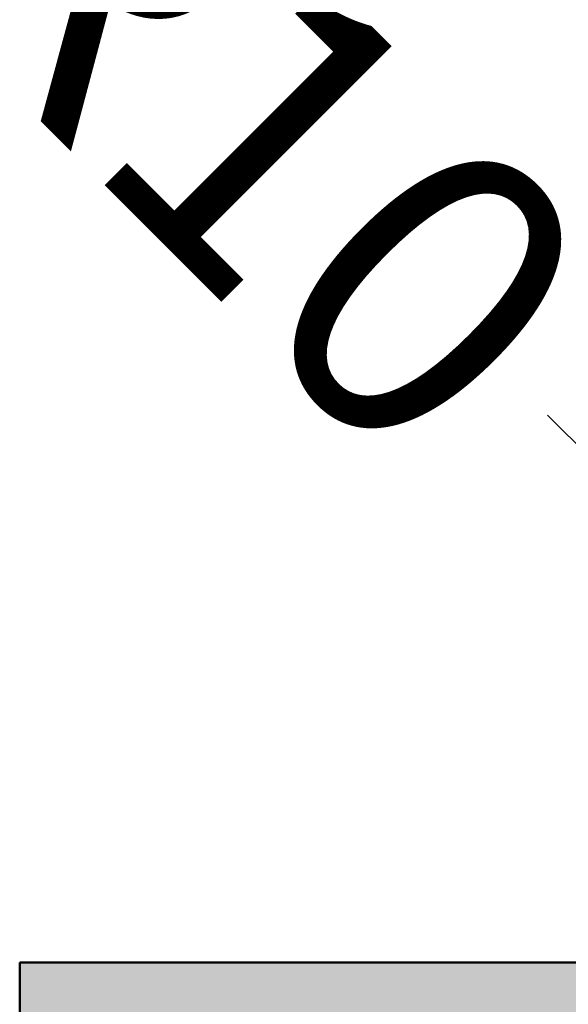
# Model space of a CAD drawing. Units: millimetres. Extents: x 0 to 2267, y 0 to 1823.
# Tile 13 of 256: x 1506 to 1519, y 1116 to 1139. Entities that reach past the tile are written whole.
import ezdxf

# ---------------------------------------------------------------- set-up
doc = ezdxf.new("R2010")
doc.units = ezdxf.units.MM
doc.header["$MEASUREMENT"] = 0
for name, color, linetype, lineweight in [('M-DIMS', 2, 'Continuous', 25), ('M-HATC', 252, 'Continuous', 18), ('M-OUTL', 7, 'Continuous', 50)]:
    doc.layers.add(name, color=color, linetype=linetype, lineweight=lineweight)
doc.styles.get("Standard").update_dxf_attribs({"font": 'arial.ttf'})
doc.dimstyles.get("Standard").update_dxf_attribs({"dimtxt": 7, "dimasz": 4, "dimexe": 0.18, "dimexo": 0.0625, "dimgap": 0.09, "dimtad": 0, "dimdec": 0, "dimzin": 0, "dimdsep": 46, "dimtxsty": 'Standard', "dimcen": 0.09, "dimadec": 0, "dimazin": 0, "dimtfac": 1, "dimtdec": 0, "dimtofl": 0, "dimtmove": 0, "dimatfit": 3, "dimfxl": 1, "dimtolj": 1, "dimtzin": 0, "dimarcsym": 0})

# ---------------------------------------------------------------- blocks, each defined once
blk = doc.blocks.new('*D28')
at = {"layer": 'Defpoints', "color": 0, "transparency": 16777216}
for p in [(1523.858, 1124.488), (1530.929, 1117.417)]:
    blk.add_point(p, dxfattribs=at)
at = {"layer": 'M-DIMS', "color": 0, "lineweight": -2, "transparency": 16777216}
for p, q in [((1518.201, 1130.145), (1521.029, 1127.317)), ((1530.839, 1117.417), (1531.019, 1117.417)), ((1530.929, 1117.327), (1530.929, 1117.507))]:
    blk.add_line(p, q, dxfattribs=at)
at = {"layer": 'M-DIMS', "color": 0, "transparency": 16777216}
blk.add_solid([(1521.501, 1127.788), (1520.558, 1126.845), (1523.858, 1124.488)], dxfattribs=at)
at = {"layer": 'M-DIMS', "color": 0, "transparency": 16777216, "insert": (1504.949, 1143.397), "char_height": 7, "attachment_point": 5, "rotation": 314.9998}
blk.add_mtext('\\A1;27X R10', dxfattribs=at)

msp = doc.modelspace()

# ---------------------------------------------------------------- hatches: boundary and pattern name
at = {"layer": 'M-HATC'}
h = msp.add_hatch(color=256, dxfattribs=at)
h.dxf.hatch_style = 1
h.paths.add_polyline_path([(2065.771, 1618.062, 0.236068), (2055.771, 1638.062), (1381.087, 1638.062, 0.236068), (1371.087, 1618.062), (1371.087, 1603.062), (2055.771, 1603.062), (2065.771, 1603.062)])
h.paths.add_polyline_path([(2062.772, 1550.296), (2062.772, 1560.296), (1374.086, 1560.296), (1374.086, 1550.296), (1374.086, 1540.296), (1384.086, 1540.296), (1389.086, 1540.296), (2062.772, 1540.296)])
h.paths.add_polyline_path([(1930.929, 1282.766), (1505.929, 1282.766), (1587.628, 1235.597, 0.131652), (1600.128, 1232.247), (1836.73, 1232.247, 0.131652), (1849.23, 1235.597)])
h.paths.add_polyline_path([(1930.929, 1117.417), (1905.929, 1117.417), (1505.929, 1117.417), (1505.929, 1077.417), (1930.929, 1077.417)])
h = msp.add_hatch(color=256, dxfattribs=at)
h.dxf.hatch_style = 1
h.paths.add_polyline_path([(2055.771, 1603.062), (1381.087, 1603.062), (1381.087, 1598.062), (2055.771, 1598.062)])
h.paths.add_polyline_path([(2055.771, 1598.062), (1381.087, 1598.062), (1381.087, 1593.062), (2055.771, 1593.062)])
h.paths.add_polyline_path([(2051.307, 1536.761), (1385.55, 1536.761), (1385.55, 1526.761), (1387.55, 1526.761), (1388.537, 1525.053), (1385.332, 1521.233), (1385.332, 1521.223), (2050.254, 1522.749), (2048.321, 1525.053), (2049.307, 1526.761), (2051.307, 1526.761)])
edge = h.paths.add_edge_path()
edge.add_arc((1847.535, 1379.149), 135, 222.60306, 222.89085, ccw=False)
edge.add_line((1748.166, 1287.766), (1683.092, 1287.766))
edge.add_arc((1583.724, 1379.149), 135, 317.10915, 317.39694, ccw=False)
edge.add_arc((1678.969, 1290.671), 5, 222.8909, 317.1091, ccw=False)
edge.add_arc((1774.213, 1379.149), 135, 222.60306, 222.89085, ccw=False)
edge.add_line((1674.845, 1287.766), (1609.771, 1287.766))
edge.add_arc((1510.403, 1379.149), 135, 317.10915, 317.39694, ccw=False)
edge.add_arc((1605.647, 1290.671), 5, 222.8909, 317.1091, ccw=False)
edge.add_arc((1700.892, 1379.149), 135, 222.60306, 222.89085, ccw=False)
edge.add_line((1601.524, 1287.766), (1536.45, 1287.766))
edge.add_arc((1437.081, 1379.149), 135, 317.10915, 317.39694, ccw=False)
edge.add_arc((1532.326, 1290.671), 5, 222.8909, 317.1091, ccw=False)
edge.add_arc((1627.571, 1379.149), 135, 222.60306, 222.89085, ccw=False)
edge.add_line((1528.203, 1287.766), (1505.929, 1287.766))
edge.add_spline(control_points=[(1505.929, 1287.766), (1504.262, 1287.766), (1504.262, 1282.766), (1505.929, 1282.766)], knot_values=[0, 0, 0, 0, 5, 5, 5, 5], degree=3, periodic=0)
edge.add_line((1505.929, 1282.766), (1930.929, 1282.766))
edge.add_spline(control_points=[(1930.929, 1282.766), (1932.596, 1282.766), (1932.596, 1287.766), (1930.929, 1287.766)], knot_values=[0, 0, 0, 0, 5, 5, 5, 5], degree=3, periodic=0)
edge.add_line((1930.929, 1287.766), (1903.056, 1287.766))
edge.add_arc((1803.688, 1379.149), 135, 317.10915, 317.39694, ccw=False)
edge.add_arc((1898.932, 1290.671), 5, 222.8909, 317.1091, ccw=False)
edge.add_arc((1994.177, 1379.149), 135, 222.60306, 222.89085, ccw=False)
edge.add_line((1894.809, 1287.766), (1829.735, 1287.766))
edge.add_arc((1730.366, 1379.149), 135, 317.10915, 317.39694, ccw=False)
edge.add_arc((1825.611, 1290.671), 5, 222.8909, 317.1091, ccw=False)
edge.add_arc((1920.856, 1379.149), 135, 222.60306, 222.89085, ccw=False)
edge.add_line((1821.487, 1287.766), (1756.413, 1287.766))
edge.add_arc((1657.045, 1379.149), 135, 317.10915, 317.39694, ccw=False)
edge.add_arc((1752.29, 1290.671), 5, 222.8909, 317.1091, ccw=False)
edge = h.paths.add_edge_path()
edge.add_spline(control_points=[(1843.429, 1227.247), (1845.096, 1227.247), (1845.096, 1232.247), (1843.429, 1232.247)], knot_values=[0, 0, 0, 0, 5, 5, 5, 5], degree=3, periodic=0)
edge.add_line((1843.429, 1232.247), (1593.429, 1232.247))
edge.add_spline(control_points=[(1593.429, 1232.247), (1591.762, 1232.247), (1591.762, 1227.247), (1593.429, 1227.247)], knot_values=[0, 0, 0, 0, 5, 5, 5, 5], degree=3, periodic=0)
edge.add_line((1593.429, 1227.247), (1843.429, 1227.247))
h.paths.add_polyline_path([(1905.929, 1127.417), (1530.929, 1127.417, 0.414214), (1520.929, 1117.417), (1530.929, 1117.417), (1915.929, 1117.417, 0.414214)])
edge = h.paths.add_edge_path()
edge.add_arc((1397.086, 1498.408), 12.73, 90.7821, 190.8787, ccw=False)
edge.add_line((1396.912, 1511.136), (1428.01, 1511.349))
edge.add_line((1428.01, 1511.349), (1433.01, 1511.349))
edge.add_line((1433.01, 1511.349), (1434.439, 1511.349))
edge.add_arc((1419.474, 1498.08), 20, 41.561, 74.0821)
edge.add_line((1424.959, 1517.314), (1399.935, 1517.256))
edge.add_spline(control_points=[(1399.931, 1517.256), (1399.884, 1517.213), (1399.833, 1517.169), (1399.777, 1517.124)], knot_values=[11.567499, 11.567499, 11.567499, 11.567499, 11.814249, 11.814249, 11.814249, 11.814249], degree=3, periodic=0)
edge.add_spline(control_points=[(1399.633, 1517.01), (1399.583, 1516.972), (1399.531, 1516.934), (1399.476, 1516.895)], knot_values=[11.167718, 11.167718, 11.167718, 11.167718, 11.365188, 11.365188, 11.365188, 11.365188], degree=3, periodic=0)
edge.add_spline(control_points=[(1399.34, 1516.8), (1399.151, 1516.672), (1398.938, 1516.538), (1398.704, 1516.399)], knot_values=[10.376405, 10.376405, 10.376405, 10.376405, 11.00994, 11.00994, 11.00994, 11.00994], degree=3, periodic=0)
edge.add_spline(control_points=[(1398.657, 1516.372), (1398.579, 1516.326), (1398.498, 1516.28), (1398.415, 1516.233)], knot_values=[10.125175, 10.125175, 10.125175, 10.125175, 10.334406, 10.334406, 10.334406, 10.334406], degree=3, periodic=0)
edge.add_spline(control_points=[(1398.264, 1516.149), (1398.196, 1516.111), (1398.126, 1516.073), (1398.055, 1516.035)], knot_values=[9.832246, 9.832246, 9.832246, 9.832246, 9.999658, 9.999658, 9.999658, 9.999658], degree=3, periodic=0)
edge.add_spline(control_points=[(1397.999, 1516.005), (1397.731, 1515.862), (1397.446, 1515.717), (1397.147, 1515.571)], knot_values=[9.161808, 9.161808, 9.161808, 9.161808, 9.787769, 9.787769, 9.787769, 9.787769], degree=3, periodic=0)
edge.add_spline(control_points=[(1397.147, 1515.571), (1396.842, 1515.423), (1396.522, 1515.274), (1396.191, 1515.126)], knot_values=[8.524455, 8.524455, 8.524455, 8.524455, 9.161808, 9.161808, 9.161808, 9.161808], degree=3, periodic=0)
edge.add_spline(control_points=[(1396.078, 1515.076), (1395.985, 1515.035), (1395.892, 1514.994), (1395.798, 1514.953)], knot_values=[8.275193, 8.275193, 8.275193, 8.275193, 8.451726, 8.451726, 8.451726, 8.451726], degree=3, periodic=0)
edge.add_spline(control_points=[(1395.602, 1514.869), (1395.5, 1514.826), (1395.397, 1514.782), (1395.293, 1514.739)], knot_values=[7.962917, 7.962917, 7.962917, 7.962917, 8.152764, 8.152764, 8.152764, 8.152764], degree=3, periodic=0)
edge.add_spline(control_points=[(1395.212, 1514.706), (1394.828, 1514.547), (1394.435, 1514.393), (1394.036, 1514.244)], knot_values=[7.21254, 7.21254, 7.21254, 7.21254, 7.913148, 7.913148, 7.913148, 7.913148], degree=3, periodic=0)
edge.add_spline(control_points=[(1394.036, 1514.244), (1393.708, 1514.121), (1393.375, 1514.003), (1393.043, 1513.889)], knot_values=[6.633733, 6.633733, 6.633733, 6.633733, 7.21254, 7.21254, 7.21254, 7.21254], degree=3, periodic=0)
edge.add_spline(control_points=[(1392.821, 1513.815), (1392.72, 1513.781), (1392.618, 1513.748), (1392.517, 1513.715)], knot_values=[6.328796, 6.328796, 6.328796, 6.328796, 6.505493, 6.505493, 6.505493, 6.505493], degree=3, periodic=0)
edge.add_spline(control_points=[(1392.517, 1513.715), (1392.319, 1513.652), (1392.121, 1513.59), (1391.924, 1513.531)], knot_values=[5.984605, 5.984605, 5.984605, 5.984605, 6.328796, 6.328796, 6.328796, 6.328796], degree=3, periodic=0)
edge.add_spline(control_points=[(1391.792, 1513.491), (1391.312, 1513.35), (1390.838, 1513.224), (1390.378, 1513.117)], knot_values=[5.066697, 5.066697, 5.066697, 5.066697, 5.907055, 5.907055, 5.907055, 5.907055], degree=3, periodic=0)
edge.add_spline(control_points=[(1390.378, 1513.117), (1390.18, 1513.071), (1389.984, 1513.028), (1389.791, 1512.99)], knot_values=[4.70367, 4.70367, 4.70367, 4.70367, 5.066695, 5.066695, 5.066695, 5.066695], degree=3, periodic=0)
edge.add_spline(control_points=[(1389.422, 1512.92), (1389.246, 1512.889), (1389.073, 1512.862), (1388.904, 1512.838)], knot_values=[4.130571, 4.130571, 4.130571, 4.130571, 4.469816, 4.469816, 4.469816, 4.469816], degree=3, periodic=0)
edge.add_spline(control_points=[(1388.904, 1512.838), (1388.591, 1512.795), (1388.291, 1512.764), (1388.007, 1512.749)], knot_values=[3.504031, 3.504031, 3.504031, 3.504031, 4.130571, 4.130571, 4.130571, 4.130571], degree=3, periodic=0)
edge.add_spline(control_points=[(1387.936, 1512.746), (1387.854, 1512.742), (1387.773, 1512.74), (1387.694, 1512.739)], knot_values=[3.268866, 3.268866, 3.268866, 3.268866, 3.451164, 3.451164, 3.451164, 3.451164], degree=3, periodic=0)
edge.add_spline(control_points=[(1387.335, 1512.744), (1387.208, 1512.75), (1387.085, 1512.76), (1386.967, 1512.774)], knot_values=[2.670686, 2.670686, 2.670686, 2.670686, 2.984, 2.984, 2.984, 2.984], degree=3, periodic=0)
edge.add_spline(control_points=[(1386.833, 1512.792), (1386.821, 1512.794), (1386.809, 1512.796), (1386.797, 1512.798)], knot_values=[2.516981, 2.516981, 2.516981, 2.516981, 2.549528, 2.549528, 2.549528, 2.549528], degree=3, periodic=0)
edge.add_spline(control_points=[(1386.453, 1512.873), (1386.426, 1512.881), (1386.399, 1512.889), (1386.373, 1512.897)], knot_values=[2.095869, 2.095869, 2.095869, 2.095869, 2.17941, 2.17941, 2.17941, 2.17941], degree=3, periodic=0)
edge.add_spline(control_points=[(1386.069, 1513.019), (1386.063, 1513.022), (1386.058, 1513.025), (1386.052, 1513.028)], knot_values=[1.72453, 1.72453, 1.72453, 1.72453, 1.745933, 1.745933, 1.745933, 1.745933], degree=3, periodic=0)
edge.add_arc((1399.474, 1498.08), 20, 131.8243, 180)
edge.add_arc((1630.334, 1505.548), 250.971, 181.70518, 236.42798)
edge.add_arc((1605.34, 1483.304), 218.782, 238.66083, 243.34961)
edge.add_arc((1647.091, 1510.359), 262.899, 183.12984, 237.85344, ccw=False)
h.paths.add_polyline_path([(1406.537, 1391.964, 0.149382), (1491.551, 1296.442, -0.129517)], flags=17)
edge = h.paths.add_edge_path()
edge.add_arc((2037.384, 1498.08), 20, 0, 48.2659)
edge.add_spline(control_points=[(2050.697, 1513.005), (2050.651, 1512.985), (2050.603, 1512.966), (2050.554, 1512.948)], knot_values=[1.835652, 1.835652, 1.835652, 1.835652, 2.000781, 2.000781, 2.000781, 2.000781], degree=3, periodic=0)
edge.add_spline(control_points=[(2050.462, 1512.917), (2050.479, 1512.922), (2050.496, 1512.928), (2050.513, 1512.934)], knot_values=[2.045477, 2.045477, 2.045477, 2.045477, 2.101389, 2.101389, 2.101389, 2.101389], degree=3, periodic=0)
edge.add_spline(control_points=[(2050.129, 1512.834), (2050.198, 1512.847), (2050.266, 1512.862), (2050.331, 1512.879)], knot_values=[2.237629, 2.237629, 2.237629, 2.237629, 2.435841, 2.435841, 2.435841, 2.435841], degree=3, periodic=0)
edge.add_spline(control_points=[(2050.095, 1512.828), (2050.106, 1512.83), (2050.118, 1512.832), (2050.129, 1512.834)], knot_values=[2.435841, 2.435841, 2.435841, 2.435841, 2.468321, 2.468321, 2.468321, 2.468321], degree=3, periodic=0)
edge.add_spline(control_points=[(2049.784, 1512.785), (2049.855, 1512.792), (2049.924, 1512.801), (2049.992, 1512.811)], knot_values=[2.563852, 2.563852, 2.563852, 2.563852, 2.748541, 2.748541, 2.748541, 2.748541], degree=3, periodic=0)
edge.add_spline(control_points=[(2049.405, 1512.762), (2049.536, 1512.765), (2049.663, 1512.773), (2049.784, 1512.785)], knot_values=[2.748541, 2.748541, 2.748541, 2.748541, 3.064882, 3.064882, 3.064882, 3.064882], degree=3, periodic=0)
edge.add_spline(control_points=[(2049.17, 1512.76), (2049.234, 1512.759), (2049.297, 1512.759), (2049.358, 1512.761)], knot_values=[3.102309, 3.102309, 3.102309, 3.102309, 3.2503, 3.2503, 3.2503, 3.2503], degree=3, periodic=0)
edge.add_spline(control_points=[(2048.857, 1512.769), (2048.964, 1512.764), (2049.068, 1512.761), (2049.17, 1512.76)], knot_values=[3.2503, 3.2503, 3.2503, 3.2503, 3.486069, 3.486069, 3.486069, 3.486069], degree=3, periodic=0)
edge.add_spline(control_points=[(2048.692, 1512.779), (2048.373, 1512.801), (2048.035, 1512.841), (2047.682, 1512.897)], knot_values=[3.606429, 3.606429, 3.606429, 3.606429, 4.2989, 4.2989, 4.2989, 4.2989], degree=3, periodic=0)
edge.add_spline(control_points=[(2047.682, 1512.897), (2047.546, 1512.919), (2047.408, 1512.942), (2047.268, 1512.969)], knot_values=[4.2989, 4.2989, 4.2989, 4.2989, 4.565769, 4.565769, 4.565769, 4.565769], degree=3, periodic=0)
edge.add_spline(control_points=[(2047.268, 1512.969), (2047.145, 1512.991), (2047.021, 1513.016), (2046.895, 1513.042)], knot_values=[4.565769, 4.565769, 4.565769, 4.565769, 4.799971, 4.799971, 4.799971, 4.799971], degree=3, periodic=0)
edge.add_spline(control_points=[(2046.895, 1513.042), (2046.529, 1513.119), (2046.151, 1513.209), (2045.768, 1513.311)], knot_values=[4.799971, 4.799971, 4.799971, 4.799971, 5.483718, 5.483718, 5.483718, 5.483718], degree=3, periodic=0)
edge.add_spline(control_points=[(2045.768, 1513.311), (2045.372, 1513.415), (2044.97, 1513.532), (2044.566, 1513.659)], knot_values=[5.483718, 5.483718, 5.483718, 5.483718, 6.187866, 6.187866, 6.187866, 6.187866], degree=3, periodic=0)
edge.add_spline(control_points=[(2044.566, 1513.659), (2044.415, 1513.706), (2044.263, 1513.755), (2044.112, 1513.805)], knot_values=[6.187866, 6.187866, 6.187866, 6.187866, 6.451551, 6.451551, 6.451551, 6.451551], degree=3, periodic=0)
edge.add_spline(control_points=[(2044.112, 1513.805), (2043.997, 1513.843), (2043.882, 1513.881), (2043.767, 1513.92)], knot_values=[6.451551, 6.451551, 6.451551, 6.451551, 6.651434, 6.651434, 6.651434, 6.651434], degree=3, periodic=0)
edge.add_spline(control_points=[(2043.767, 1513.92), (2043.372, 1514.055), (2042.977, 1514.198), (2042.589, 1514.346)], knot_values=[6.651434, 6.651434, 6.651434, 6.651434, 7.338879, 7.338879, 7.338879, 7.338879], degree=3, periodic=0)
edge.add_spline(control_points=[(2042.589, 1514.346), (2042.164, 1514.507), (2041.746, 1514.675), (2041.341, 1514.846)], knot_values=[7.338879, 7.338879, 7.338879, 7.338879, 8.089209, 8.089209, 8.089209, 8.089209], degree=3, periodic=0)
edge.add_spline(control_points=[(2041.341, 1514.846), (2041.103, 1514.946), (2040.869, 1515.048), (2040.64, 1515.15)], knot_values=[8.089209, 8.089209, 8.089209, 8.089209, 8.529587, 8.529587, 8.529587, 8.529587], degree=3, periodic=0)
edge.add_spline(control_points=[(2040.51, 1515.209), (2040.082, 1515.402), (2039.675, 1515.597), (2039.295, 1515.789)], knot_values=[8.613818, 8.613818, 8.613818, 8.613818, 9.44571, 9.44571, 9.44571, 9.44571], degree=3, periodic=0)
edge.add_spline(control_points=[(2039.295, 1515.789), (2039.062, 1515.907), (2038.839, 1516.025), (2038.629, 1516.14)], knot_values=[9.44571, 9.44571, 9.44571, 9.44571, 9.956404, 9.956404, 9.956404, 9.956404], degree=3, periodic=0)
edge.add_spline(control_points=[(2038.629, 1516.14), (2038.519, 1516.2), (2038.412, 1516.26), (2038.309, 1516.319)], knot_values=[9.956404, 9.956404, 9.956404, 9.956404, 10.223542, 10.223542, 10.223542, 10.223542], degree=3, periodic=0)
edge.add_spline(control_points=[(2038.309, 1516.319), (2038.214, 1516.374), (2038.122, 1516.428), (2038.033, 1516.481)], knot_values=[10.223542, 10.223542, 10.223542, 10.223542, 10.47051, 10.47051, 10.47051, 10.47051], degree=3, periodic=0)
edge.add_spline(control_points=[(2038.033, 1516.481), (2037.786, 1516.63), (2037.564, 1516.773), (2037.372, 1516.909)], knot_values=[10.47051, 10.47051, 10.47051, 10.47051, 11.15767, 11.15767, 11.15767, 11.15767], degree=3, periodic=0)
edge.add_spline(control_points=[(2037.372, 1516.909), (2037.279, 1516.975), (2037.193, 1517.04), (2037.114, 1517.102)], knot_values=[11.15767, 11.15767, 11.15767, 11.15767, 11.49227, 11.49227, 11.49227, 11.49227], degree=3, periodic=0)
edge.add_spline(control_points=[(2036.856, 1517.326), (2036.915, 1517.269), (2036.981, 1517.21), (2037.056, 1517.149)], knot_values=[11.577341, 11.577341, 11.577341, 11.577341, 11.91035, 11.91035, 11.91035, 11.91035], degree=3, periodic=0)
edge.add_spline(control_points=[(2036.807, 1517.375), (2036.823, 1517.359), (2036.839, 1517.342), (2036.856, 1517.326)], knot_values=[11.91035, 11.91035, 11.91035, 11.91035, 12.007402, 12.007402, 12.007402, 12.007402], degree=3, periodic=0)
edge.add_spline(control_points=[(2036.702, 1517.494), (2036.71, 1517.483), (2036.72, 1517.472), (2036.729, 1517.461)], knot_values=[12.184155, 12.184155, 12.184155, 12.184155, 12.255409, 12.255409, 12.255409, 12.255409], degree=3, periodic=0)
edge.add_spline(control_points=[(2036.616, 1517.621), (2036.62, 1517.613), (2036.624, 1517.606), (2036.629, 1517.598)], knot_values=[12.487913, 12.487913, 12.487913, 12.487913, 12.541035, 12.541035, 12.541035, 12.541035], degree=3, periodic=0)
edge.add_spline(control_points=[(2036.563, 1517.786), (2036.564, 1517.779), (2036.564, 1517.773), (2036.565, 1517.766)], knot_values=[12.911761, 12.911761, 12.911761, 12.911761, 12.968286, 12.968286, 12.968286, 12.968286], degree=3, periodic=0)
edge.add_spline(control_points=[(2036.617, 1517.93), (2036.612, 1517.926), (2036.609, 1517.921), (2036.605, 1517.916)], knot_values=[13.382527, 13.382527, 13.382527, 13.382527, 13.433791, 13.433791, 13.433791, 13.433791], degree=3, periodic=0)
edge.add_spline(control_points=[(2036.749, 1518.017), (2036.736, 1518.012), (2036.724, 1518.006), (2036.712, 1518)], knot_values=[13.726299, 13.726299, 13.726299, 13.726299, 13.809928, 13.809928, 13.809928, 13.809928], degree=3, periodic=0)
edge.add_spline(control_points=[(2036.86, 1518.053), (2036.839, 1518.047), (2036.818, 1518.042), (2036.799, 1518.035)], knot_values=[13.910887, 13.910887, 13.910887, 13.910887, 14.02153, 14.02153, 14.02153, 14.02153], degree=3, periodic=0)
edge.add_line((2036.964, 1518.08), (2032.384, 1518.08))
edge.add_line((2032.384, 1518.08), (2027.384, 1518.08))
edge.add_line((2027.384, 1518.08), (2022.384, 1518.08))
edge.add_line((2022.384, 1518.08), (2017.384, 1518.08))
edge.add_arc((2017.384, 1498.08), 20, 90, 138.439)
edge.add_line((2002.419, 1511.349), (2003.848, 1511.349))
edge.add_line((2003.848, 1511.349), (2008.848, 1511.349))
edge.add_line((2008.848, 1511.349), (2039.772, 1511.138))
edge.add_arc((2039.772, 1498.408), 12.73, -10.8787, 90, ccw=False)
edge.add_arc((1789.767, 1510.359), 262.899, 302.14656, 356.87016, ccw=False)
edge.add_arc((1831.518, 1483.304), 218.782, 296.65039, 301.33917)
edge.add_arc((1806.524, 1505.548), 250.971, 303.57202, 358.29482)
h.paths.add_polyline_path([(2030.321, 1391.964, -0.129517), (1945.307, 1296.442, 0.149382)], flags=17)
edge = h.paths.add_edge_path()
edge.add_spline(control_points=[(2037.246, 1518.082), (2037.29, 1518.081), (2037.336, 1518.08), (2037.384, 1518.08)], knot_values=[0.000012, 0.000012, 0.000012, 0.000012, 0.144754, 0.144754, 0.144754, 0.144754], degree=3, periodic=0)
edge.add_line((2037.336, 1518.08), (2037.01, 1518.08))
edge.add_spline(control_points=[(2037.01, 1518.08), (2036.982, 1518.077), (2036.956, 1518.073), (2036.931, 1518.068)], knot_values=[14.13465, 14.13465, 14.13465, 14.13465, 14.247197, 14.247197, 14.247197, 14.247197], degree=3, periodic=0)
edge.add_spline(control_points=[(2036.931, 1518.068), (2036.928, 1518.067), (2036.924, 1518.067), (2036.921, 1518.066)], knot_values=[14.118315, 14.118315, 14.118315, 14.118315, 14.13465, 14.13465, 14.13465, 14.13465], degree=3, periodic=0)
edge.add_spline(control_points=[(2036.921, 1518.066), (2036.912, 1518.064), (2036.903, 1518.063), (2036.895, 1518.061)], knot_values=[14.078086, 14.078086, 14.078086, 14.078086, 14.118315, 14.118315, 14.118315, 14.118315], degree=3, periodic=0)
edge.add_spline(control_points=[(2036.895, 1518.061), (2036.883, 1518.058), (2036.872, 1518.056), (2036.86, 1518.053)], knot_values=[14.02153, 14.02153, 14.02153, 14.02153, 14.078086, 14.078086, 14.078086, 14.078086], degree=3, periodic=0)
edge.add_spline(control_points=[(2036.86, 1518.053), (2036.839, 1518.047), (2036.818, 1518.042), (2036.799, 1518.035)], knot_values=[13.910887, 13.910887, 13.910887, 13.910887, 14.02153, 14.02153, 14.02153, 14.02153], degree=3, periodic=0)
edge.add_spline(control_points=[(2036.799, 1518.035), (2036.798, 1518.035), (2036.797, 1518.035), (2036.797, 1518.035)], knot_values=[13.906906, 13.906906, 13.906906, 13.906906, 13.910887, 13.910887, 13.910887, 13.910887], degree=3, periodic=0)
edge.add_spline(control_points=[(2036.797, 1518.035), (2036.788, 1518.032), (2036.78, 1518.029), (2036.772, 1518.026)], knot_values=[13.857826, 13.857826, 13.857826, 13.857826, 13.906906, 13.906906, 13.906906, 13.906906], degree=3, periodic=0)
edge.add_spline(control_points=[(2036.772, 1518.026), (2036.764, 1518.023), (2036.756, 1518.02), (2036.749, 1518.017)], knot_values=[13.809928, 13.809928, 13.809928, 13.809928, 13.857826, 13.857826, 13.857826, 13.857826], degree=3, periodic=0)
edge.add_spline(control_points=[(2036.749, 1518.017), (2036.736, 1518.012), (2036.724, 1518.006), (2036.712, 1518)], knot_values=[13.726299, 13.726299, 13.726299, 13.726299, 13.809928, 13.809928, 13.809928, 13.809928], degree=3, periodic=0)
edge.add_spline(control_points=[(2036.712, 1518), (2036.712, 1518), (2036.712, 1518), (2036.711, 1518)], knot_values=[13.723993, 13.723993, 13.723993, 13.723993, 13.726299, 13.726299, 13.726299, 13.726299], degree=3, periodic=0)
edge.add_spline(control_points=[(2036.711, 1518), (2036.706, 1517.997), (2036.701, 1517.994), (2036.696, 1517.992)], knot_values=[13.686536, 13.686536, 13.686536, 13.686536, 13.723993, 13.723993, 13.723993, 13.723993], degree=3, periodic=0)
edge.add_spline(control_points=[(2036.696, 1517.992), (2036.692, 1517.989), (2036.687, 1517.987), (2036.683, 1517.984)], knot_values=[13.651251, 13.651251, 13.651251, 13.651251, 13.686536, 13.686536, 13.686536, 13.686536], degree=3, periodic=0)
edge.add_spline(control_points=[(2036.683, 1517.984), (2036.676, 1517.98), (2036.67, 1517.976), (2036.664, 1517.971)], knot_values=[13.596804, 13.596804, 13.596804, 13.596804, 13.651251, 13.651251, 13.651251, 13.651251], degree=3, periodic=0)
edge.add_spline(control_points=[(2036.664, 1517.971), (2036.664, 1517.971), (2036.663, 1517.971), (2036.663, 1517.971)], knot_values=[13.593956, 13.593956, 13.593956, 13.593956, 13.596804, 13.596804, 13.596804, 13.596804], degree=3, periodic=0)
edge.add_spline(control_points=[(2036.663, 1517.971), (2036.66, 1517.969), (2036.658, 1517.967), (2036.655, 1517.965)], knot_values=[13.570322, 13.570322, 13.570322, 13.570322, 13.593956, 13.593956, 13.593956, 13.593956], degree=3, periodic=0)
edge.add_spline(control_points=[(2036.655, 1517.965), (2036.653, 1517.963), (2036.65, 1517.961), (2036.647, 1517.959)], knot_values=[13.545477, 13.545477, 13.545477, 13.545477, 13.570322, 13.570322, 13.570322, 13.570322], degree=3, periodic=0)
edge.add_spline(control_points=[(2036.647, 1517.959), (2036.647, 1517.959), (2036.647, 1517.959), (2036.647, 1517.959)], knot_values=[13.543931, 13.543931, 13.543931, 13.543931, 13.545477, 13.545477, 13.545477, 13.545477], degree=3, periodic=0)
edge.add_spline(control_points=[(2036.647, 1517.959), (2036.641, 1517.954), (2036.636, 1517.949), (2036.631, 1517.945)], knot_values=[13.488237, 13.488237, 13.488237, 13.488237, 13.543931, 13.543931, 13.543931, 13.543931], degree=3, periodic=0)
edge.add_spline(control_points=[(2036.631, 1517.945), (2036.628, 1517.942), (2036.626, 1517.94), (2036.623, 1517.937)], knot_values=[13.460307, 13.460307, 13.460307, 13.460307, 13.488237, 13.488237, 13.488237, 13.488237], degree=3, periodic=0)
edge.add_spline(control_points=[(2036.623, 1517.937), (2036.622, 1517.936), (2036.62, 1517.934), (2036.618, 1517.932)], knot_values=[13.439712, 13.439712, 13.439712, 13.439712, 13.460307, 13.460307, 13.460307, 13.460307], degree=3, periodic=0)
edge.add_spline(control_points=[(2036.618, 1517.932), (2036.618, 1517.931), (2036.617, 1517.931), (2036.617, 1517.93)], knot_values=[13.433791, 13.433791, 13.433791, 13.433791, 13.439712, 13.439712, 13.439712, 13.439712], degree=3, periodic=0)
edge.add_spline(control_points=[(2036.617, 1517.93), (2036.612, 1517.926), (2036.609, 1517.921), (2036.605, 1517.916)], knot_values=[13.382527, 13.382527, 13.382527, 13.382527, 13.433791, 13.433791, 13.433791, 13.433791], degree=3, periodic=0)
edge.add_spline(control_points=[(2036.605, 1517.916), (2036.603, 1517.913), (2036.6, 1517.91), (2036.598, 1517.907)], knot_values=[13.350017, 13.350017, 13.350017, 13.350017, 13.382527, 13.382527, 13.382527, 13.382527], degree=3, periodic=0)
edge.add_spline(control_points=[(2036.598, 1517.907), (2036.597, 1517.906), (2036.596, 1517.904), (2036.595, 1517.903)], knot_values=[13.333922, 13.333922, 13.333922, 13.333922, 13.350017, 13.350017, 13.350017, 13.350017], degree=3, periodic=0)
edge.add_spline(control_points=[(2036.595, 1517.903), (2036.595, 1517.902), (2036.594, 1517.901), (2036.593, 1517.9)], knot_values=[13.323828, 13.323828, 13.323828, 13.323828, 13.333922, 13.333922, 13.333922, 13.333922], degree=3, periodic=0)
edge.add_spline(control_points=[(2036.593, 1517.9), (2036.59, 1517.895), (2036.588, 1517.891), (2036.585, 1517.886)], knot_values=[13.277545, 13.277545, 13.277545, 13.277545, 13.323828, 13.323828, 13.323828, 13.323828], degree=3, periodic=0)
edge.add_spline(control_points=[(2036.585, 1517.886), (2036.584, 1517.883), (2036.582, 1517.879), (2036.58, 1517.875)], knot_values=[13.240119, 13.240119, 13.240119, 13.240119, 13.277545, 13.277545, 13.277545, 13.277545], degree=3, periodic=0)
edge.add_spline(control_points=[(2036.58, 1517.875), (2036.58, 1517.874), (2036.579, 1517.873), (2036.578, 1517.872)], knot_values=[13.228211, 13.228211, 13.228211, 13.228211, 13.240119, 13.240119, 13.240119, 13.240119], degree=3, periodic=0)
edge.add_spline(control_points=[(2036.578, 1517.872), (2036.578, 1517.87), (2036.577, 1517.869), (2036.577, 1517.868)], knot_values=[13.215717, 13.215717, 13.215717, 13.215717, 13.228211, 13.228211, 13.228211, 13.228211], degree=3, periodic=0)
edge.add_spline(control_points=[(2036.577, 1517.868), (2036.575, 1517.864), (2036.574, 1517.86), (2036.573, 1517.857)], knot_values=[13.179847, 13.179847, 13.179847, 13.179847, 13.215717, 13.215717, 13.215717, 13.215717], degree=3, periodic=0)
edge.add_spline(control_points=[(2036.573, 1517.857), (2036.571, 1517.851), (2036.57, 1517.846), (2036.569, 1517.841)], knot_values=[13.132017, 13.132017, 13.132017, 13.132017, 13.179847, 13.179847, 13.179847, 13.179847], degree=3, periodic=0)
edge.add_spline(control_points=[(2036.569, 1517.841), (2036.568, 1517.84), (2036.568, 1517.839), (2036.568, 1517.838)], knot_values=[13.122482, 13.122482, 13.122482, 13.122482, 13.132017, 13.132017, 13.132017, 13.132017], degree=3, periodic=0)
edge.add_spline(control_points=[(2036.568, 1517.838), (2036.568, 1517.836), (2036.567, 1517.835), (2036.567, 1517.833)], knot_values=[13.105592, 13.105592, 13.105592, 13.105592, 13.122482, 13.122482, 13.122482, 13.122482], degree=3, periodic=0)
edge.add_spline(control_points=[(2036.567, 1517.833), (2036.566, 1517.829), (2036.566, 1517.826), (2036.565, 1517.822)], knot_values=[13.074063, 13.074063, 13.074063, 13.074063, 13.105592, 13.105592, 13.105592, 13.105592], degree=3, periodic=0)
edge.add_spline(control_points=[(2036.565, 1517.822), (2036.565, 1517.822), (2036.565, 1517.822), (2036.565, 1517.822)], knot_values=[13.074043, 13.074043, 13.074043, 13.074043, 13.074063, 13.074063, 13.074063, 13.074063], degree=3, periodic=0)
edge.add_spline(control_points=[(2036.565, 1517.822), (2036.564, 1517.816), (2036.564, 1517.811), (2036.564, 1517.805)], knot_values=[13.021884, 13.021884, 13.021884, 13.021884, 13.074043, 13.074043, 13.074043, 13.074043], degree=3, periodic=0)
edge.add_spline(control_points=[(2036.564, 1517.805), (2036.564, 1517.804), (2036.564, 1517.803), (2036.564, 1517.803)], knot_values=[13.01674, 13.01674, 13.01674, 13.01674, 13.021884, 13.021884, 13.021884, 13.021884], degree=3, periodic=0)
edge.add_spline(control_points=[(2036.564, 1517.803), (2036.563, 1517.801), (2036.563, 1517.798), (2036.563, 1517.796)], knot_values=[12.996438, 12.996438, 12.996438, 12.996438, 13.01674, 13.01674, 13.01674, 13.01674], degree=3, periodic=0)
edge.add_spline(control_points=[(2036.563, 1517.796), (2036.563, 1517.793), (2036.563, 1517.789), (2036.563, 1517.786)], knot_values=[12.968286, 12.968286, 12.968286, 12.968286, 12.996438, 12.996438, 12.996438, 12.996438], degree=3, periodic=0)
edge.add_spline(control_points=[(2036.563, 1517.786), (2036.564, 1517.779), (2036.564, 1517.773), (2036.565, 1517.766)], knot_values=[12.911761, 12.911761, 12.911761, 12.911761, 12.968286, 12.968286, 12.968286, 12.968286], degree=3, periodic=0)
edge.add_spline(control_points=[(2036.565, 1517.766), (2036.565, 1517.766), (2036.565, 1517.766), (2036.565, 1517.766)], knot_values=[12.911017, 12.911017, 12.911017, 12.911017, 12.911761, 12.911761, 12.911761, 12.911761], degree=3, periodic=0)
edge.add_spline(control_points=[(2036.565, 1517.766), (2036.565, 1517.762), (2036.566, 1517.759), (2036.566, 1517.756)], knot_values=[12.88528, 12.88528, 12.88528, 12.88528, 12.911017, 12.911017, 12.911017, 12.911017], degree=3, periodic=0)
edge.add_spline(control_points=[(2036.566, 1517.756), (2036.567, 1517.753), (2036.567, 1517.751), (2036.568, 1517.748)], knot_values=[12.862519, 12.862519, 12.862519, 12.862519, 12.88528, 12.88528, 12.88528, 12.88528], degree=3, periodic=0)
edge.add_spline(control_points=[(2036.568, 1517.748), (2036.568, 1517.747), (2036.568, 1517.747), (2036.568, 1517.746)], knot_values=[12.858885, 12.858885, 12.858885, 12.858885, 12.862519, 12.862519, 12.862519, 12.862519], degree=3, periodic=0)
edge.add_spline(control_points=[(2036.568, 1517.746), (2036.569, 1517.74), (2036.571, 1517.733), (2036.572, 1517.726)], knot_values=[12.8053, 12.8053, 12.8053, 12.8053, 12.858885, 12.858885, 12.858885, 12.858885], degree=3, periodic=0)
edge.add_spline(control_points=[(2036.572, 1517.726), (2036.573, 1517.723), (2036.574, 1517.719), (2036.576, 1517.715)], knot_values=[12.775176, 12.775176, 12.775176, 12.775176, 12.8053, 12.8053, 12.8053, 12.8053], degree=3, periodic=0)
edge.add_spline(control_points=[(2036.576, 1517.715), (2036.576, 1517.713), (2036.577, 1517.71), (2036.578, 1517.708)], knot_values=[12.756759, 12.756759, 12.756759, 12.756759, 12.775176, 12.775176, 12.775176, 12.775176], degree=3, periodic=0)
edge.add_spline(control_points=[(2036.578, 1517.708), (2036.578, 1517.707), (2036.578, 1517.706), (2036.579, 1517.705)], knot_values=[12.748742, 12.748742, 12.748742, 12.748742, 12.756759, 12.756759, 12.756759, 12.756759], degree=3, periodic=0)
edge.add_spline(control_points=[(2036.579, 1517.705), (2036.581, 1517.698), (2036.583, 1517.692), (2036.586, 1517.685)], knot_values=[12.69959, 12.69959, 12.69959, 12.69959, 12.748742, 12.748742, 12.748742, 12.748742], degree=3, periodic=0)
edge.add_spline(control_points=[(2036.586, 1517.685), (2036.588, 1517.68), (2036.59, 1517.675), (2036.592, 1517.669)], knot_values=[12.659038, 12.659038, 12.659038, 12.659038, 12.69959, 12.69959, 12.69959, 12.69959], degree=3, periodic=0)
edge.add_spline(control_points=[(2036.592, 1517.669), (2036.594, 1517.665), (2036.596, 1517.66), (2036.598, 1517.656)], knot_values=[12.626806, 12.626806, 12.626806, 12.626806, 12.659038, 12.659038, 12.659038, 12.659038], degree=3, periodic=0)
edge.add_spline(control_points=[(2036.598, 1517.656), (2036.598, 1517.655), (2036.599, 1517.654), (2036.599, 1517.653)], knot_values=[12.619394, 12.619394, 12.619394, 12.619394, 12.626806, 12.626806, 12.626806, 12.626806], degree=3, periodic=0)
edge.add_spline(control_points=[(2036.599, 1517.653), (2036.604, 1517.642), (2036.61, 1517.632), (2036.616, 1517.621)], knot_values=[12.541039, 12.541039, 12.541039, 12.541039, 12.619394, 12.619394, 12.619394, 12.619394], degree=3, periodic=0)
edge.add_spline(control_points=[(2036.616, 1517.621), (2036.616, 1517.621), (2036.616, 1517.621), (2036.616, 1517.621)], knot_values=[12.541035, 12.541035, 12.541035, 12.541035, 12.541039, 12.541039, 12.541039, 12.541039], degree=3, periodic=0)
edge.add_spline(control_points=[(2036.616, 1517.621), (2036.62, 1517.613), (2036.624, 1517.606), (2036.629, 1517.598)], knot_values=[12.487913, 12.487913, 12.487913, 12.487913, 12.541035, 12.541035, 12.541035, 12.541035], degree=3, periodic=0)
edge.add_spline(control_points=[(2036.629, 1517.598), (2036.633, 1517.592), (2036.637, 1517.585), (2036.641, 1517.579)], knot_values=[12.443982, 12.443982, 12.443982, 12.443982, 12.487913, 12.487913, 12.487913, 12.487913], degree=3, periodic=0)
edge.add_spline(control_points=[(2036.641, 1517.579), (2036.641, 1517.578), (2036.642, 1517.576), (2036.643, 1517.575)], knot_values=[12.434996, 12.434996, 12.434996, 12.434996, 12.443982, 12.443982, 12.443982, 12.443982], degree=3, periodic=0)
edge.add_spline(control_points=[(2036.643, 1517.575), (2036.653, 1517.56), (2036.664, 1517.544), (2036.676, 1517.528)], knot_values=[12.329647, 12.329647, 12.329647, 12.329647, 12.434996, 12.434996, 12.434996, 12.434996], degree=3, periodic=0)
edge.add_spline(control_points=[(2036.676, 1517.528), (2036.684, 1517.517), (2036.693, 1517.505), (2036.702, 1517.494)], knot_values=[12.255409, 12.255409, 12.255409, 12.255409, 12.329647, 12.329647, 12.329647, 12.329647], degree=3, periodic=0)
edge.add_spline(control_points=[(2036.702, 1517.494), (2036.71, 1517.483), (2036.72, 1517.472), (2036.729, 1517.461)], knot_values=[12.184155, 12.184155, 12.184155, 12.184155, 12.255409, 12.255409, 12.255409, 12.255409], degree=3, periodic=0)
edge.add_spline(control_points=[(2036.729, 1517.461), (2036.744, 1517.444), (2036.759, 1517.426), (2036.775, 1517.409)], knot_values=[12.075961, 12.075961, 12.075961, 12.075961, 12.184155, 12.184155, 12.184155, 12.184155], degree=3, periodic=0)
edge.add_spline(control_points=[(2036.775, 1517.409), (2036.776, 1517.407), (2036.777, 1517.406), (2036.778, 1517.405)], knot_values=[12.069502, 12.069502, 12.069502, 12.069502, 12.075961, 12.075961, 12.075961, 12.075961], degree=3, periodic=0)
edge.add_spline(control_points=[(2036.778, 1517.405), (2036.788, 1517.395), (2036.797, 1517.385), (2036.807, 1517.375)], knot_values=[12.007402, 12.007402, 12.007402, 12.007402, 12.069502, 12.069502, 12.069502, 12.069502], degree=3, periodic=0)
edge.add_spline(control_points=[(2036.807, 1517.375), (2036.823, 1517.359), (2036.839, 1517.342), (2036.856, 1517.326)], knot_values=[11.91035, 11.91035, 11.91035, 11.91035, 12.007402, 12.007402, 12.007402, 12.007402], degree=3, periodic=0)
edge.add_spline(control_points=[(2036.856, 1517.326), (2036.915, 1517.269), (2036.981, 1517.21), (2037.056, 1517.149)], knot_values=[11.577341, 11.577341, 11.577341, 11.577341, 11.91035, 11.91035, 11.91035, 11.91035], degree=3, periodic=0)
edge.add_spline(control_points=[(2037.056, 1517.149), (2037.075, 1517.134), (2037.094, 1517.118), (2037.114, 1517.102)], knot_values=[11.49227, 11.49227, 11.49227, 11.49227, 11.577341, 11.577341, 11.577341, 11.577341], degree=3, periodic=0)
edge.add_spline(control_points=[(2037.114, 1517.102), (2037.193, 1517.04), (2037.279, 1516.975), (2037.372, 1516.909)], knot_values=[11.15767, 11.15767, 11.15767, 11.15767, 11.49227, 11.49227, 11.49227, 11.49227], degree=3, periodic=0)
edge.add_spline(control_points=[(2037.372, 1516.909), (2037.564, 1516.773), (2037.786, 1516.63), (2038.033, 1516.481)], knot_values=[10.47051, 10.47051, 10.47051, 10.47051, 11.15767, 11.15767, 11.15767, 11.15767], degree=3, periodic=0)
edge.add_spline(control_points=[(2038.033, 1516.481), (2038.122, 1516.428), (2038.214, 1516.374), (2038.309, 1516.319)], knot_values=[10.223542, 10.223542, 10.223542, 10.223542, 10.47051, 10.47051, 10.47051, 10.47051], degree=3, periodic=0)
edge.add_spline(control_points=[(2038.309, 1516.319), (2038.412, 1516.26), (2038.519, 1516.2), (2038.629, 1516.14)], knot_values=[9.956404, 9.956404, 9.956404, 9.956404, 10.223542, 10.223542, 10.223542, 10.223542], degree=3, periodic=0)
edge.add_spline(control_points=[(2038.629, 1516.14), (2038.839, 1516.025), (2039.062, 1515.907), (2039.295, 1515.789)], knot_values=[9.44571, 9.44571, 9.44571, 9.44571, 9.956404, 9.956404, 9.956404, 9.956404], degree=3, periodic=0)
edge.add_spline(control_points=[(2039.295, 1515.789), (2039.675, 1515.597), (2040.082, 1515.402), (2040.51, 1515.209)], knot_values=[8.613818, 8.613818, 8.613818, 8.613818, 9.44571, 9.44571, 9.44571, 9.44571], degree=3, periodic=0)
edge.add_spline(control_points=[(2040.51, 1515.209), (2040.553, 1515.189), (2040.597, 1515.17), (2040.64, 1515.15)], knot_values=[8.529587, 8.529587, 8.529587, 8.529587, 8.613818, 8.613818, 8.613818, 8.613818], degree=3, periodic=0)
edge.add_spline(control_points=[(2040.64, 1515.15), (2040.869, 1515.048), (2041.103, 1514.946), (2041.341, 1514.846)], knot_values=[8.089209, 8.089209, 8.089209, 8.089209, 8.529587, 8.529587, 8.529587, 8.529587], degree=3, periodic=0)
edge.add_spline(control_points=[(2041.341, 1514.846), (2041.746, 1514.675), (2042.164, 1514.507), (2042.589, 1514.346)], knot_values=[7.338879, 7.338879, 7.338879, 7.338879, 8.089209, 8.089209, 8.089209, 8.089209], degree=3, periodic=0)
edge.add_spline(control_points=[(2042.589, 1514.346), (2042.977, 1514.198), (2043.372, 1514.055), (2043.767, 1513.92)], knot_values=[6.651434, 6.651434, 6.651434, 6.651434, 7.338879, 7.338879, 7.338879, 7.338879], degree=3, periodic=0)
edge.add_spline(control_points=[(2043.767, 1513.92), (2043.882, 1513.881), (2043.997, 1513.843), (2044.112, 1513.805)], knot_values=[6.451551, 6.451551, 6.451551, 6.451551, 6.651434, 6.651434, 6.651434, 6.651434], degree=3, periodic=0)
edge.add_spline(control_points=[(2044.112, 1513.805), (2044.263, 1513.755), (2044.415, 1513.706), (2044.566, 1513.659)], knot_values=[6.187866, 6.187866, 6.187866, 6.187866, 6.451551, 6.451551, 6.451551, 6.451551], degree=3, periodic=0)
edge.add_spline(control_points=[(2044.566, 1513.659), (2044.97, 1513.532), (2045.372, 1513.415), (2045.768, 1513.311)], knot_values=[5.483718, 5.483718, 5.483718, 5.483718, 6.187866, 6.187866, 6.187866, 6.187866], degree=3, periodic=0)
edge.add_spline(control_points=[(2045.768, 1513.311), (2046.151, 1513.209), (2046.529, 1513.119), (2046.895, 1513.042)], knot_values=[4.799971, 4.799971, 4.799971, 4.799971, 5.483718, 5.483718, 5.483718, 5.483718], degree=3, periodic=0)
edge.add_spline(control_points=[(2046.895, 1513.042), (2047.021, 1513.016), (2047.145, 1512.991), (2047.268, 1512.969)], knot_values=[4.565769, 4.565769, 4.565769, 4.565769, 4.799971, 4.799971, 4.799971, 4.799971], degree=3, periodic=0)
edge.add_spline(control_points=[(2047.268, 1512.969), (2047.408, 1512.942), (2047.546, 1512.919), (2047.682, 1512.897)], knot_values=[4.2989, 4.2989, 4.2989, 4.2989, 4.565769, 4.565769, 4.565769, 4.565769], degree=3, periodic=0)
edge.add_spline(control_points=[(2047.682, 1512.897), (2048.035, 1512.841), (2048.373, 1512.801), (2048.692, 1512.779)], knot_values=[3.606429, 3.606429, 3.606429, 3.606429, 4.2989, 4.2989, 4.2989, 4.2989], degree=3, periodic=0)
edge.add_spline(control_points=[(2048.692, 1512.779), (2048.748, 1512.775), (2048.803, 1512.772), (2048.857, 1512.769)], knot_values=[3.486069, 3.486069, 3.486069, 3.486069, 3.606429, 3.606429, 3.606429, 3.606429], degree=3, periodic=0)
edge.add_spline(control_points=[(2048.857, 1512.769), (2048.964, 1512.764), (2049.068, 1512.761), (2049.17, 1512.76)], knot_values=[3.2503, 3.2503, 3.2503, 3.2503, 3.486069, 3.486069, 3.486069, 3.486069], degree=3, periodic=0)
edge.add_spline(control_points=[(2049.17, 1512.76), (2049.234, 1512.759), (2049.297, 1512.759), (2049.358, 1512.761)], knot_values=[3.102309, 3.102309, 3.102309, 3.102309, 3.2503, 3.2503, 3.2503, 3.2503], degree=3, periodic=0)
edge.add_spline(control_points=[(2049.358, 1512.761), (2049.374, 1512.761), (2049.39, 1512.761), (2049.405, 1512.762)], knot_values=[3.064882, 3.064882, 3.064882, 3.064882, 3.102309, 3.102309, 3.102309, 3.102309], degree=3, periodic=0)
edge.add_spline(control_points=[(2049.405, 1512.762), (2049.536, 1512.765), (2049.663, 1512.773), (2049.784, 1512.785)], knot_values=[2.748541, 2.748541, 2.748541, 2.748541, 3.064882, 3.064882, 3.064882, 3.064882], degree=3, periodic=0)
edge.add_spline(control_points=[(2049.784, 1512.785), (2049.855, 1512.792), (2049.924, 1512.801), (2049.992, 1512.811)], knot_values=[2.563852, 2.563852, 2.563852, 2.563852, 2.748541, 2.748541, 2.748541, 2.748541], degree=3, periodic=0)
edge.add_spline(control_points=[(2049.992, 1512.811), (2050.026, 1512.816), (2050.061, 1512.822), (2050.095, 1512.828)], knot_values=[2.468321, 2.468321, 2.468321, 2.468321, 2.563852, 2.563852, 2.563852, 2.563852], degree=3, periodic=0)
edge.add_spline(control_points=[(2050.095, 1512.828), (2050.106, 1512.83), (2050.118, 1512.832), (2050.129, 1512.834)], knot_values=[2.435841, 2.435841, 2.435841, 2.435841, 2.468321, 2.468321, 2.468321, 2.468321], degree=3, periodic=0)
edge.add_spline(control_points=[(2050.129, 1512.834), (2050.198, 1512.847), (2050.266, 1512.862), (2050.331, 1512.879)], knot_values=[2.237629, 2.237629, 2.237629, 2.237629, 2.435841, 2.435841, 2.435841, 2.435841], degree=3, periodic=0)
edge.add_spline(control_points=[(2050.331, 1512.879), (2050.375, 1512.891), (2050.419, 1512.903), (2050.462, 1512.917)], knot_values=[2.101389, 2.101389, 2.101389, 2.101389, 2.237629, 2.237629, 2.237629, 2.237629], degree=3, periodic=0)
edge.add_spline(control_points=[(2050.462, 1512.917), (2050.479, 1512.922), (2050.496, 1512.928), (2050.513, 1512.934)], knot_values=[2.045477, 2.045477, 2.045477, 2.045477, 2.101389, 2.101389, 2.101389, 2.101389], degree=3, periodic=0)
edge.add_spline(control_points=[(2050.513, 1512.934), (2050.527, 1512.938), (2050.54, 1512.943), (2050.554, 1512.948)], knot_values=[2.000781, 2.000781, 2.000781, 2.000781, 2.045477, 2.045477, 2.045477, 2.045477], degree=3, periodic=0)
edge.add_spline(control_points=[(2050.554, 1512.948), (2050.603, 1512.966), (2050.651, 1512.985), (2050.697, 1513.005)], knot_values=[1.835652, 1.835652, 1.835652, 1.835652, 2.000781, 2.000781, 2.000781, 2.000781], degree=3, periodic=0)
edge.add_arc((2037.384, 1498.08), 20, 48.2659, 90.1299)
edge = h.paths.add_edge_path(flags=16)
edge.add_spline(control_points=[(1386.139, 1512.986), (1388.92, 1511.739), (1398.039, 1515.519), (1399.931, 1517.256)], knot_values=[1.831046, 1.831046, 1.831046, 1.831046, 11.814249, 11.814249, 11.814249, 11.814249], degree=3, periodic=0)
edge.add_line((1399.931, 1517.256), (1393.743, 1517.242))
edge.add_arc((1399.474, 1498.08), 20, 106.6501, 131.8173)

# ---------------------------------------------------------------- linework, layer by layer
at = {"layer": 'M-OUTL'}
for q in [(1930.929, 1117.417), (1505.929, 1077.417), (1530.929, 1117.417)]:
    msp.add_line((1505.929, 1117.417), q, dxfattribs=at)

# ---------------------------------------------------------------- dimensions: what is measured, and where the dimension line sits
at = {"layer": 'M-DIMS'}
dim = msp.add_radius_dim(center=(1530.929, 1117.417), mpoint=(1523.858, 1124.488), text='27X <>', dimstyle='Standard', override={"dimdec": 0, "dimlfac": 1, "dimrnd": 0, "dimzin": 0, "dimdsep": 46, "dimlunit": 2}, dxfattribs=at)
dim.commit()
dim.dimension.update_dxf_attribs({"geometry": '*D28', "text_midpoint": (1504.949, 1143.397)})

doc.saveas('drawing.dxf')
